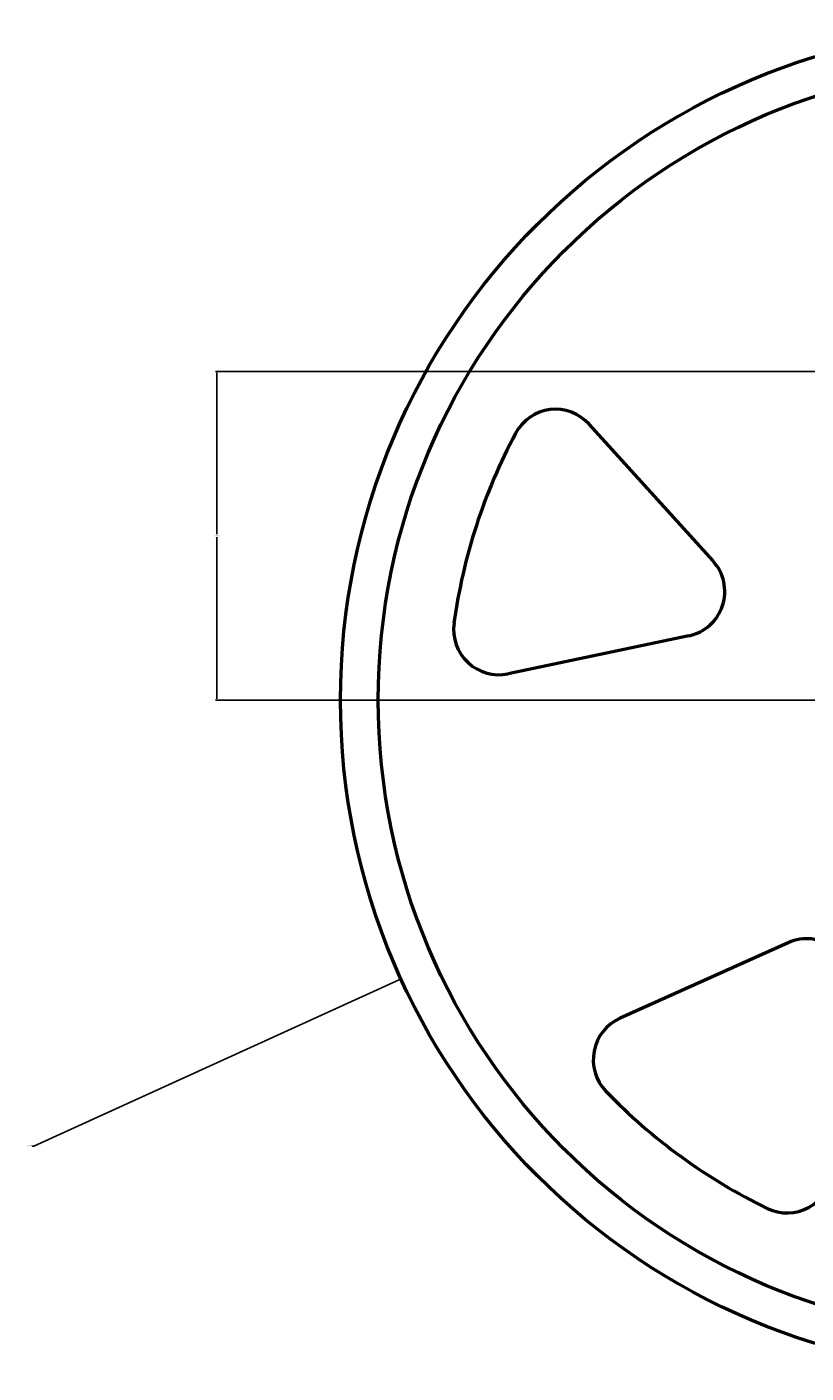
# Model space of a CAD drawing. Units: inches. Extents: x -99 to 284, y -92 to 134.
# Tile 1 of 16: x -99 to 5, y -74 to 104. Entities that reach past the tile are written whole.
import ezdxf

# ---------------------------------------------------------------- set-up
doc = ezdxf.new("R2010")
doc.units = ezdxf.units.IN
doc.header["$MEASUREMENT"] = 0
doc.layers.add('M-DIMS', color=2, linetype='Continuous', lineweight=18)
doc.layers.add('M-OUTL', color=7, linetype='Continuous', lineweight=50)
doc.styles.get("Standard").update_dxf_attribs({"font": 'arial.ttf'})
doc.dimstyles.get("Standard").update_dxf_attribs({"dimtxt": 0.18, "dimasz": 0.18, "dimexe": 0.18, "dimexo": 0.0625, "dimgap": 0.09, "dimtad": 0, "dimtih": 1, "dimtoh": 1, "dimdec": 4, "dimzin": 0, "dimdsep": 46, "dimtxsty": 'Standard', "dimcen": 0.09, "dimadec": 0, "dimazin": 0, "dimtfac": 1, "dimtdec": 4, "dimtofl": 0, "dimtmove": 0, "dimatfit": 3, "dimfxl": 1, "dimtolj": 1, "dimtzin": 0, "dimarcsym": 0})

# ---------------------------------------------------------------- blocks, each defined once
blk = doc.blocks.new('*U1')
for p, q in [((-5.21, -13.52), (-17.34, 7.65)), ((5.21, -13.52), (17.34, 7.65))]:
    blk.add_line(p, q)
for centre, start, end in [((-12.14, 10.63), 100.177, 209.8264), ((12.14, 10.63), 330.1736, 79.823), ((0, -10.54), 209.8264, 330.1736)]:
    blk.add_arc(centre, 6, start, end)
blk = doc.blocks.new('*U2')
at = {"layer": 'M-OUTL', "color": 0, "linetype": 'ByBlock', "lineweight": -2, "transparency": 16777216}
blk.add_blockref('*U1', (31.98, 71.82), dxfattribs=at)
for p, rotation in [((-22.2, 32.46), 72), ((86.16, 32.46), 288), ((-1.51, -31.24), 144), ((65.46, -31.24), 216)]:
    blk.add_blockref('*U1', p, dxfattribs=dict(at, rotation=rotation))
blk = doc.blocks.new('*D9')
at = {"layer": 'Defpoints', "color": 0, "transparency": 16777216}
for p in [(26.77, 58.3), (-73.37, 14.85), (31.98, 14.85)]:
    blk.add_point(p, dxfattribs=at)
at = {"layer": 'M-DIMS', "color": 0, "lineweight": -2, "transparency": 16777216}
for p, q in [((26.71, 58.3), (-73.55, 58.3)), ((-73.37, 58.12), (-73.37, 36.76)), ((-73.37, 15.03), (-73.37, 36.4)), ((31.91, 14.85), (-73.55, 14.85))]:
    blk.add_line(p, q, dxfattribs=at)
at = {"layer": 'M-DIMS', "color": 0, "transparency": 16777216}
for points in [[(-73.4, 58.12), (-73.34, 58.12), (-73.37, 58.3)], [(-73.4, 15.03), (-73.34, 15.03), (-73.37, 14.85)]]:
    blk.add_solid(points, dxfattribs=at)
at = {"layer": 'M-DIMS', "color": 0, "transparency": 16777216, "insert": (-73.37, 36.58), "char_height": 0.18, "attachment_point": 5}
blk.add_mtext('\\A1;43.45', dxfattribs=at)
blk = doc.blocks.new('*D19')
at = {"layer": 'Defpoints', "color": 0, "transparency": 16777216}
for p in [(112.98, 51.72), (-49.03, -22.01)]:
    blk.add_point(p, dxfattribs=at)
at = {"layer": 'M-DIMS', "color": 0, "lineweight": -2, "transparency": 16777216}
for p, q in [((31.89, 14.85), (32.07, 14.85)), ((31.98, 14.76), (31.98, 14.94)), ((-97.63, -44.13), (-49.19, -22.09)), ((-97.81, -44.13), (-97.63, -44.13))]:
    blk.add_line(p, q, dxfattribs=at)
at = {"layer": 'M-DIMS', "color": 0, "transparency": 16777216}
blk.add_solid([(-49.2, -22.06), (-49.18, -22.11), (-49.03, -22.01)], dxfattribs=at)
at = {"layer": 'M-DIMS', "color": 0, "transparency": 16777216, "insert": (-98.2, -44.13), "char_height": 0.18, "attachment_point": 5}
blk.add_mtext('\\A1;∅178', dxfattribs=at)
blk = doc.blocks.new('*D20')
at = {"layer": 'Defpoints', "color": 0, "transparency": 16777216}
for p in [(-35.23, 65.25), (99.18, -35.54)]:
    blk.add_point(p, dxfattribs=at)
at = {"layer": 'M-DIMS', "color": 0, "lineweight": -2, "transparency": 16777216}
for p, q in [((31.89, 14.85), (32.07, 14.85)), ((31.98, 14.76), (31.98, 14.94)), ((139.51, -65.77), (99.33, -35.65)), ((139.69, -65.77), (139.51, -65.77))]:
    blk.add_line(p, q, dxfattribs=at)
at = {"layer": 'M-DIMS', "color": 0, "transparency": 16777216}
blk.add_solid([(99.35, -35.62), (99.31, -35.67), (99.18, -35.54)], dxfattribs=at)
at = {"layer": 'M-DIMS', "color": 0, "transparency": 16777216, "insert": (140.07, -65.77), "char_height": 0.18, "attachment_point": 5}
blk.add_mtext('\\A1;∅168', dxfattribs=at)

msp = doc.modelspace()

# ---------------------------------------------------------------- linework, layer by layer
at = {"layer": 'M-OUTL'}
for radius in [89, 84]:
    msp.add_circle((31.9765, 14.8539), radius, dxfattribs=at)
for start, end in [(151.823035, 172.176965), (223.823035, 244.176965)]:
    msp.add_arc((31.9765, 14.8539), 74.6806, start, end, dxfattribs=at)

# ---------------------------------------------------------------- block references
msp.add_blockref('*U2', (0, 0), dxfattribs=at)

# ---------------------------------------------------------------- dimensions: what is measured, and where the dimension line sits
at = {"layer": 'M-DIMS'}
for p1, p2, picture, middle in [((-35.2301, 65.2451), (99.1831, -35.5373), '*D20', (140.074, -65.772)), ((112.9816, 51.7208), (-49.0286, -22.013), '*D19', (-98.1987, -44.1332))]:
    dim = msp.add_diameter_dim_2p(p1=p1, p2=p2, dimstyle='Standard', override={"dimdec": 0, "dimlfac": 1, "dimrnd": 0, "dimzin": 0, "dimdsep": 46, "dimlunit": 2}, dxfattribs=at)
    dim.commit()
    dim.dimension.update_dxf_attribs({"geometry": picture, "text_midpoint": middle, "dimtype": 163})
dim = msp.add_linear_dim(base=(-73.3735, 14.8539), p1=(26.7713, 58.3032), p2=(31.9765, 14.8539), angle=90, dimstyle='Standard', override={"dimdec": 2, "dimlfac": 1, "dimrnd": 0, "dimzin": 0, "dimdsep": 46, "dimlunit": 2}, dxfattribs=at)
dim.commit()
dim.dimension.update_dxf_attribs({"geometry": '*D9', "text_midpoint": (-73.3735, 36.5785)})

doc.saveas('drawing.dxf')
